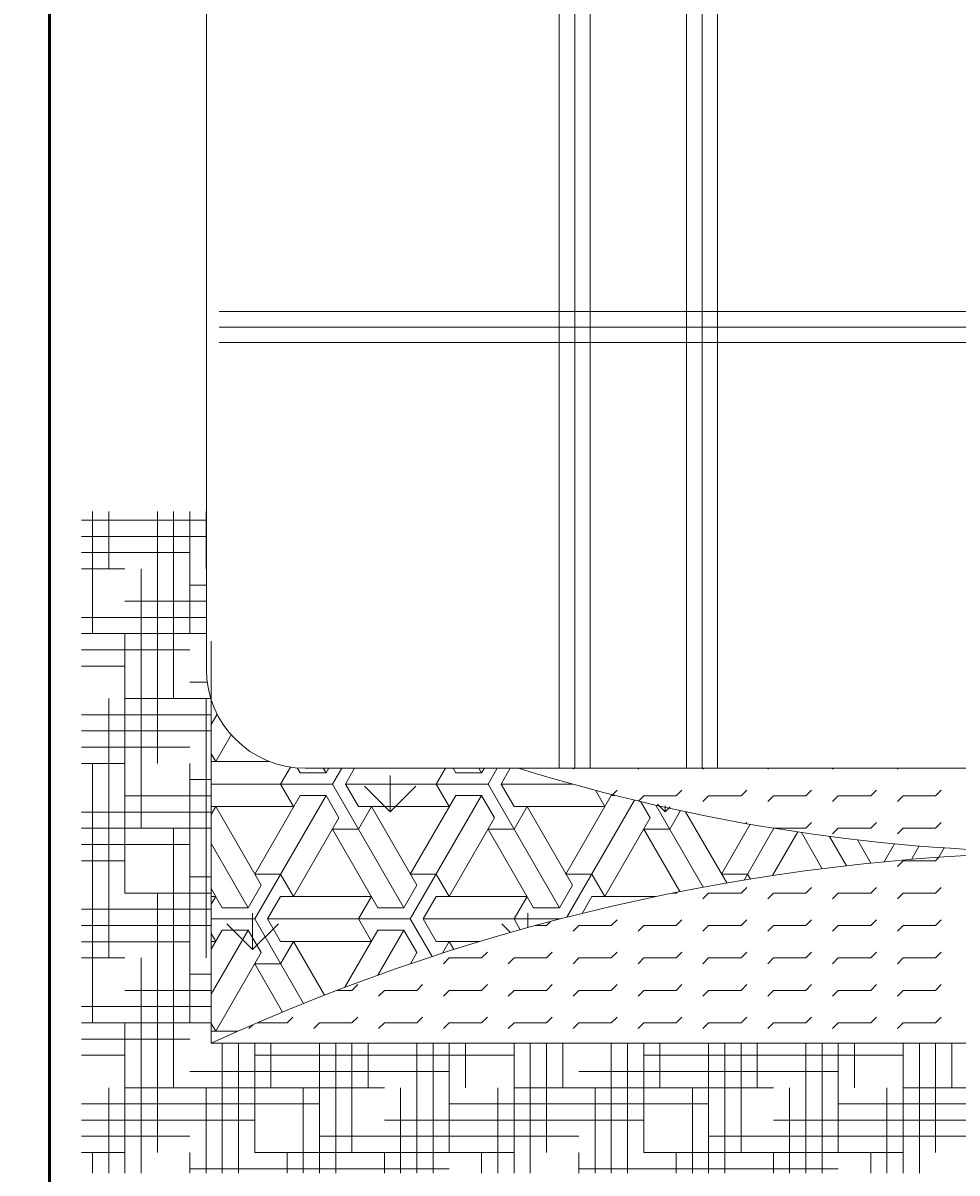
# Model space of a CAD drawing. Units: inches. Extents: x -1517 to -668, y -425 to 52.
# Tile 8 of 13: x -1186 to -1161, y -63 to -32. Entities that reach past the tile are written whole.
import ezdxf

# ---------------------------------------------------------------- set-up
doc = ezdxf.new("R2010")
doc.units = ezdxf.units.IN
doc.header["$MEASUREMENT"] = 0
for name, color, linetype, lineweight in [('A-ANNO-DIMS', 2, 'Continuous', 18), ('furniture block', 8, 'Continuous', 18), ('walls', 240, 'Continuous', 50)]:
    doc.layers.add(name, color=color, linetype=linetype, lineweight=lineweight)
doc.styles.get("Standard").update_dxf_attribs({"font": 'arial.ttf'})
doc.dimstyles.get("Standard").update_dxf_attribs({"dimtxt": 0.18, "dimasz": 0.18, "dimexe": 0.18, "dimexo": 0.0625, "dimgap": 0.09, "dimtad": 0, "dimtih": 1, "dimtoh": 1, "dimdec": 4, "dimzin": 0, "dimdsep": 46, "dimlunit": 4, "dimtxsty": 'Standard', "dimcen": 0.09, "dimadec": 0, "dimazin": 0, "dimtfac": 1, "dimtdec": 4, "dimtofl": 0, "dimtmove": 0, "dimatfit": 3, "dimfxl": 1, "dimtolj": 1, "dimtzin": 0, "dimarcsym": 0})

# ---------------------------------------------------------------- blocks, each defined once
blk = doc.blocks.new('A$C62731D1C')
for p, q in [((0.09627, 0.38824, 0.68571), (0.09627, 2.14084, 0.68571)), ((0.46643, 1.44371, 0.68571), (0.46643, 0.31204, 0.68571)), ((0.47843, 1.44371, 0.68571), (0.47843, 0.31204, 0.68571)), ((0.49043, 1.44371, 0.68571), (0.49043, 0.31204, 0.68571)), ((0.36826, 1.4076, 0.68571), (0.36826, 0.31204, 0.68571)), ((0.38026, 1.4076, 0.68571), (0.38026, 0.31204, 0.68571)), ((0.39226, 1.4076, 0.68571), (0.39226, 0.31204, 0.68571)), ((0.10613, 0.66415, 0.68571), (1.46095, 0.66415, 0.68571)), ((0.10613, 0.65215, 0.68571), (1.46095, 0.65215, 0.68571)), ((0.10613, 0.64015, 0.68571), (1.46095, 0.64015, 0.68571)), ((0.0085, 0.41577, 0.68571), (0.0085, 0.50998, 0.68571)), ((0.021, 0.46577, 0.68571), (0.021, 0.50998, 0.68571)), ((0.0585, 0.31577, 0.68571), (0.0585, 0.50998, 0.68571)), ((0.071, 0.36577, 0.68571), (0.071, 0.50998, 0.68571)), ((0.0835, 0.41577, 0.68571), (0.0835, 0.50998, 0.68571)), ((0.096, 0.46577, 0.68571), (0.096, 0.50998, 0.68571)), ((0, 0.50327, 0.68571), (0.09627, 0.50327, 0.68571)), ((0, 0.49077, 0.68571), (0.09627, 0.49077, 0.68571)), ((0, 0.47827, 0.68571), (0.0835, 0.47827, 0.68571)), ((0, 0.46577, 0.68571), (0.0335, 0.46577, 0.68571)), ((0.046, 0.26577, 0.68571), (0.046, 0.46577, 0.68571)), ((0.0835, 0.45327, 0.68571), (0.09627, 0.45327, 0.68571)), ((0.0335, 0.44077, 0.68571), (0.09627, 0.44077, 0.68571)), ((0, 0.42827, 0.68571), (0.09627, 0.42827, 0.68571)), ((0, 0.41577, 0.68571), (0.09627, 0.41577, 0.68571)), ((0.0335, 0.21577, 0.68571), (0.0335, 0.41577, 0.68571)), ((0.1, 0.1, 0.68571), (0.1, 0.40998, 0.68571)), ((0, 0.40327, 0.68571), (0.0835, 0.40327, 0.68571)), ((0, 0.39077, 0.68571), (0.0335, 0.39077, 0.68571)), ((0.0835, 0.37827, 0.68571), (0.09693, 0.37827, 0.68571)), ((0.021, 0.16577, 0.68571), (0.021, 0.36577, 0.68571)), ((0.0335, 0.36577, 0.68571), (0.09966, 0.36577, 0.68571)), ((0.096, 0.16577, 0.68571), (0.096, 0.36577, 0.68571)), ((0, 0.35327, 0.68571), (0.1, 0.35327, 0.68571)), ((0.1, 0.34567, 0.68571), (0.10459, 0.35362, 0.68571)), ((0, 0.34077, 0.68571), (0.1, 0.34077, 0.68571)), ((0.11542, 0.33773, 0.68571), (0.1035, 0.31709, 0.68571)), ((0, 0.32827, 0.68571), (0.0835, 0.32827, 0.68571)), ((0.1, 0.32316, 0.68571), (0.1035, 0.31709, 0.68571)), ((0, 0.31577, 0.68571), (0.0335, 0.31577, 0.68571)), ((0.0085, 0.11577, 0.68571), (0.0085, 0.31577, 0.68571)), ((0.0835, 0.11577, 0.68571), (0.0835, 0.31577, 0.68571)), ((0.1, 0.31709, 0.68571), (0.14518, 0.31709, 0.68571)), ((0.1535, 0.29977, 0.68571), (0.16108, 0.3129, 0.68571)), ((0.1685, 0.30843, 0.68571), (0.16627, 0.31229, 0.68571)), ((1.39167, 0.31204, 0.68571), (0.17247, 0.31204, 0.68571)), ((0.18642, 0.31204, 0.68571), (0.1885, 0.30843, 0.68571)), ((0.1885, 0.30843, 0.68571), (0.19058, 0.31204, 0.68571)), ((0.1935, 0.29977, 0.68571), (0.20058, 0.31204, 0.68571)), ((0.2035, 0.29977, 0.68571), (0.21058, 0.31204, 0.68571)), ((0.2735, 0.29977, 0.68571), (0.28058, 0.31204, 0.68571)), ((0.2885, 0.30843, 0.68571), (0.28642, 0.31204, 0.68571)), ((0.30642, 0.31204, 0.68571), (0.3085, 0.30843, 0.68571)), ((0.3085, 0.30843, 0.68571), (0.31058, 0.31204, 0.68571)), ((0.3135, 0.29977, 0.68571), (0.32058, 0.31204, 0.68571)), ((0.3235, 0.29977, 0.68571), (0.33058, 0.31204, 0.68571)), ((0.37908, 0.31135, 0.68571), (0.37977, 0.31204, 0.68571)), ((0.42908, 0.31135, 0.68571), (0.42977, 0.31204, 0.68571)), ((0.47908, 0.31135, 0.68571), (0.47977, 0.31204, 0.68571)), ((0.52908, 0.31135, 0.68571), (0.52977, 0.31204, 0.68571)), ((0.57908, 0.31135, 0.68571), (0.57977, 0.31204, 0.68571)), ((0.62908, 0.31135, 0.68571), (0.62977, 0.31204, 0.68571)), ((0.0835, 0.30327, 0.68571), (0.1, 0.30327, 0.68571)), ((0.1885, 0.30843, 0.68571), (0.1685, 0.30843, 0.68571)), ((0.23796, 0.2783, 0.68571), (0.23796, 0.30643, 0.68571)), ((0.3085, 0.30843, 0.68571), (0.2885, 0.30843, 0.68571)), ((0.1935, 0.29977, 0.68571), (0.1, 0.29977, 0.68571)), ((0.1535, 0.29977, 0.68571), (0.1635, 0.28245, 0.68571)), ((0.1935, 0.29977, 0.68571), (0.2485, 0.20451, 0.68571)), ((0.3135, 0.29977, 0.68571), (0.2035, 0.29977, 0.68571)), ((0.2035, 0.29977, 0.68571), (0.2135, 0.28245, 0.68571)), ((0.23796, 0.2783, 0.68571), (0.21807, 0.29819, 0.68571)), ((0.23796, 0.2783, 0.68571), (0.25785, 0.29819, 0.68571)), ((0.2735, 0.29977, 0.68571), (0.2835, 0.28245, 0.68571)), ((0.3135, 0.29977, 0.68571), (0.3685, 0.20451, 0.68571)), ((0.37861, 0.29977, 0.68571), (0.3235, 0.29977, 0.68571)), ((0.3235, 0.29977, 0.68571), (0.3335, 0.28245, 0.68571)), ((0.39626, 0.295, 0.68571), (0.4035, 0.28245, 0.68571)), ((0.40934, 0.29161, 0.68571), (0.41292, 0.29519, 0.68571)), ((0.4585, 0.29077, 0.68571), (0.46292, 0.29519, 0.68571)), ((0.5085, 0.29077, 0.68571), (0.51292, 0.29519, 0.68571)), ((0.5585, 0.29077, 0.68571), (0.56292, 0.29519, 0.68571)), ((0.6085, 0.29077, 0.68571), (0.61292, 0.29519, 0.68571)), ((0.6585, 0.29077, 0.68571), (0.66292, 0.29519, 0.68571)), ((0.0335, 0.29077, 0.68571), (0.1, 0.29077, 0.68571)), ((0.1335, 0.19585, 0.68571), (0.1885, 0.29111, 0.68571)), ((0.1685, 0.29111, 0.68571), (0.1335, 0.23049, 0.68571)), ((0.1885, 0.29111, 0.68571), (0.1685, 0.29111, 0.68571)), ((0.1885, 0.29111, 0.68571), (0.1985, 0.27379, 0.68571)), ((0.2535, 0.19585, 0.68571), (0.3085, 0.29111, 0.68571)), ((0.2885, 0.29111, 0.68571), (0.2535, 0.23049, 0.68571)), ((0.3085, 0.29111, 0.68571), (0.2885, 0.29111, 0.68571)), ((0.3085, 0.29111, 0.68571), (0.3185, 0.27379, 0.68571)), ((0.4085, 0.29111, 0.68571), (0.3735, 0.23049, 0.68571)), ((0.37428, 0.19721, 0.68571), (0.42636, 0.2874, 0.68571)), ((0.4113, 0.29111, 0.68571), (0.4085, 0.29111, 0.68571)), ((0.4294, 0.28667, 0.68571), (0.4335, 0.29077, 0.68571)), ((0.43133, 0.28621, 0.68571), (0.4385, 0.27379, 0.68571)), ((0.4335, 0.29077, 0.68571), (0.4585, 0.29077, 0.68571)), ((0.45009, 0.2783, 0.68571), (0.44401, 0.28439, 0.68571)), ((0.47908, 0.28635, 0.68571), (0.4835, 0.29077, 0.68571)), ((0.4835, 0.29077, 0.68571), (0.5085, 0.29077, 0.68571)), ((0.52908, 0.28635, 0.68571), (0.5335, 0.29077, 0.68571)), ((0.5335, 0.29077, 0.68571), (0.5585, 0.29077, 0.68571)), ((0.57908, 0.28635, 0.68571), (0.5835, 0.29077, 0.68571)), ((0.5835, 0.29077, 0.68571), (0.6085, 0.29077, 0.68571)), ((0.62908, 0.28635, 0.68571), (0.6335, 0.29077, 0.68571)), ((0.6335, 0.29077, 0.68571), (0.6585, 0.29077, 0.68571)), ((0, 0.27827, 0.68571), (0.1, 0.27827, 0.68571)), ((0.1, 0.27639, 0.68571), (0.1035, 0.28245, 0.68571)), ((0.1, 0.28245, 0.68571), (0.1635, 0.28245, 0.68571)), ((0.1385, 0.22183, 0.68571), (0.1035, 0.28245, 0.68571)), ((0.2135, 0.26513, 0.68571), (0.2235, 0.28245, 0.68571)), ((0.2135, 0.28245, 0.68571), (0.2835, 0.28245, 0.68571)), ((0.2585, 0.22183, 0.68571), (0.2235, 0.28245, 0.68571)), ((0.3335, 0.26513, 0.68571), (0.3435, 0.28245, 0.68571)), ((0.3335, 0.28245, 0.68571), (0.4035, 0.28245, 0.68571)), ((0.3785, 0.22183, 0.68571), (0.3435, 0.28245, 0.68571)), ((0.44289, 0.28352, 0.68571), (0.47937, 0.22033, 0.68571)), ((0.45009, 0.2783, 0.68571), (0.45009, 0.28301, 0.68571)), ((0.45009, 0.2783, 0.68571), (0.45394, 0.28215, 0.68571)), ((0.4535, 0.26513, 0.68571), (0.46171, 0.27934, 0.68571)), ((0.49749, 0.22358, 0.68571), (0.4658, 0.27847, 0.68571)), ((0.1985, 0.27379, 0.68571), (0.1635, 0.21317, 0.68571)), ((0.3185, 0.27379, 0.68571), (0.2835, 0.21317, 0.68571)), ((0.4385, 0.27379, 0.68571), (0.4035, 0.21317, 0.68571)), ((0.51564, 0.26884, 0.68571), (0.4935, 0.23049, 0.68571)), ((0.51218, 0.26945, 0.68571), (0.51292, 0.27019, 0.68571)), ((0.5585, 0.26577, 0.68571), (0.56292, 0.27019, 0.68571)), ((0.6085, 0.26577, 0.68571), (0.61292, 0.27019, 0.68571)), ((0.6585, 0.26577, 0.68571), (0.66292, 0.27019, 0.68571)), ((0, 0.26577, 0.68571), (0.1, 0.26577, 0.68571)), ((0.071, 0.06577, 0.68571), (0.071, 0.26577, 0.68571)), ((0.2135, 0.26513, 0.68571), (0.1935, 0.26513, 0.68571)), ((0.2285, 0.20451, 0.68571), (0.1935, 0.26513, 0.68571)), ((0.3335, 0.26513, 0.68571), (0.3135, 0.26513, 0.68571)), ((0.3485, 0.20451, 0.68571), (0.3135, 0.26513, 0.68571)), ((0.4535, 0.26513, 0.68571), (0.4335, 0.26513, 0.68571)), ((0.46136, 0.21689, 0.68571), (0.4335, 0.26513, 0.68571)), ((0.51081, 0.22583, 0.68571), (0.53387, 0.26577, 0.68571)), ((0.55222, 0.26292, 0.68571), (0.53281, 0.2293, 0.68571)), ((0.53385, 0.26577, 0.68571), (0.5585, 0.26577, 0.68571)), ((0.57113, 0.2346, 0.68571), (0.55502, 0.2625, 0.68571)), ((0.57677, 0.25948, 0.68571), (0.58983, 0.23685, 0.68571)), ((0.57908, 0.26135, 0.68571), (0.5835, 0.26577, 0.68571)), ((0.5835, 0.26577, 0.68571), (0.6085, 0.26577, 0.68571)), ((0.62908, 0.26135, 0.68571), (0.6335, 0.26577, 0.68571)), ((0.6335, 0.26577, 0.68571), (0.6585, 0.26577, 0.68571)), ((0, 0.25327, 0.68571), (0.0835, 0.25327, 0.68571)), ((0.1, 0.25388, 0.68571), (0.1285, 0.20451, 0.68571)), ((0.60866, 0.23889, 0.68571), (0.5983, 0.25682, 0.68571)), ((0.62695, 0.25378, 0.68571), (0.61894, 0.2399, 0.68571)), ((0.64002, 0.24179, 0.68571), (0.64597, 0.25209, 0.68571)), ((0.66513, 0.25064, 0.68571), (0.66094, 0.24338, 0.68571)), ((0, 0.24077, 0.68571), (0.0335, 0.24077, 0.68571)), ((0.62908, 0.23635, 0.68571), (0.6335, 0.24077, 0.68571)), ((0.6335, 0.24077, 0.68571), (0.6585, 0.24077, 0.68571)), ((0.6585, 0.24077, 0.68571), (0.66112, 0.24339, 0.68571)), ((0.0835, 0.22827, 0.68571), (0.1, 0.22827, 0.68571)), ((0.1285, 0.20451, 0.68571), (0.1385, 0.22183, 0.68571)), ((0.1535, 0.23049, 0.68571), (0.1335, 0.23049, 0.68571)), ((0.1535, 0.23049, 0.68571), (0.1635, 0.21317, 0.68571)), ((0.2485, 0.20451, 0.68571), (0.2585, 0.22183, 0.68571)), ((0.2735, 0.23049, 0.68571), (0.2535, 0.23049, 0.68571)), ((0.2735, 0.23049, 0.68571), (0.2835, 0.21317, 0.68571)), ((0.3685, 0.20451, 0.68571), (0.3785, 0.22183, 0.68571)), ((0.3935, 0.23049, 0.68571), (0.3735, 0.23049, 0.68571)), ((0.3935, 0.23049, 0.68571), (0.4035, 0.21317, 0.68571)), ((0.5135, 0.23049, 0.68571), (0.4935, 0.23049, 0.68571)), ((0.5135, 0.23049, 0.68571), (0.51573, 0.22663, 0.68571)), ((0.0335, 0.21577, 0.68571), (0.1, 0.21577, 0.68571)), ((0.0585, 0.01577, 0.68571), (0.0585, 0.21577, 0.68571)), ((0.1085, 0.20451, 0.68571), (0.1, 0.21924, 0.68571)), ((0.1, 0.20711, 0.68571), (0.1035, 0.21317, 0.68571)), ((0.1, 0.21317, 0.68571), (0.1035, 0.21317, 0.68571)), ((0.1435, 0.19585, 0.68571), (0.1535, 0.21317, 0.68571)), ((0.1535, 0.21317, 0.68571), (0.2235, 0.21317, 0.68571)), ((0.2135, 0.19585, 0.68571), (0.2235, 0.21317, 0.68571)), ((0.2635, 0.19585, 0.68571), (0.2735, 0.21317, 0.68571)), ((0.2735, 0.21317, 0.68571), (0.3435, 0.21317, 0.68571)), ((0.3335, 0.19585, 0.68571), (0.3435, 0.21317, 0.68571)), ((0.38598, 0.20015, 0.68571), (0.3935, 0.21317, 0.68571)), ((0.3935, 0.21317, 0.68571), (0.44307, 0.21317, 0.68571)), ((0.45574, 0.21577, 0.68571), (0.4585, 0.21577, 0.68571)), ((0.4585, 0.21577, 0.68571), (0.45919, 0.21646, 0.68571)), ((0.47908, 0.21135, 0.68571), (0.4835, 0.21577, 0.68571)), ((0.4835, 0.21577, 0.68571), (0.5085, 0.21577, 0.68571)), ((0.5085, 0.21577, 0.68571), (0.51292, 0.22019, 0.68571)), ((0.52908, 0.21135, 0.68571), (0.5335, 0.21577, 0.68571)), ((0.5335, 0.21577, 0.68571), (0.5585, 0.21577, 0.68571)), ((0.5585, 0.21577, 0.68571), (0.56292, 0.22019, 0.68571)), ((0.57908, 0.21135, 0.68571), (0.5835, 0.21577, 0.68571)), ((0.5835, 0.21577, 0.68571), (0.6085, 0.21577, 0.68571)), ((0.6085, 0.21577, 0.68571), (0.61292, 0.22019, 0.68571)), ((0.62908, 0.21135, 0.68571), (0.6335, 0.21577, 0.68571)), ((0.6335, 0.21577, 0.68571), (0.6585, 0.21577, 0.68571)), ((0.6585, 0.21577, 0.68571), (0.66292, 0.22019, 0.68571)), ((0.1285, 0.20451, 0.68571), (0.1085, 0.20451, 0.68571)), ((0.2485, 0.20451, 0.68571), (0.2285, 0.20451, 0.68571)), ((0.3685, 0.20451, 0.68571), (0.3485, 0.20451, 0.68571)), ((0, 0.20327, 0.68571), (0.1, 0.20327, 0.68571)), ((0.1335, 0.19585, 0.68571), (0.1, 0.19585, 0.68571)), ((0.13189, 0.17223, 0.68571), (0.13189, 0.20036, 0.68571)), ((0.1335, 0.19585, 0.68571), (0.17113, 0.13067, 0.68571)), ((0.2535, 0.19585, 0.68571), (0.1435, 0.19585, 0.68571)), ((0.1435, 0.19585, 0.68571), (0.1535, 0.17853, 0.68571)), ((0.2135, 0.19585, 0.68571), (0.2235, 0.17853, 0.68571)), ((0.2535, 0.19585, 0.68571), (0.27024, 0.16687, 0.68571)), ((0.36902, 0.19585, 0.68571), (0.2635, 0.19585, 0.68571)), ((0.2635, 0.19585, 0.68571), (0.2735, 0.17853, 0.68571)), ((0.3335, 0.19585, 0.68571), (0.33829, 0.18757, 0.68571)), ((0.34403, 0.18916, 0.68571), (0.34403, 0.20036, 0.68571)), ((0.4085, 0.19077, 0.68571), (0.41292, 0.19519, 0.68571)), ((0.4585, 0.19077, 0.68571), (0.46292, 0.19519, 0.68571)), ((0.5085, 0.19077, 0.68571), (0.51292, 0.19519, 0.68571)), ((0.5585, 0.19077, 0.68571), (0.56292, 0.19519, 0.68571)), ((0.6085, 0.19077, 0.68571), (0.61292, 0.19519, 0.68571)), ((0.6585, 0.19077, 0.68571), (0.66292, 0.19519, 0.68571)), ((0, 0.19077, 0.68571), (0.1, 0.19077, 0.68571)), ((0.1, 0.13782, 0.68571), (0.1285, 0.18719, 0.68571)), ((0.1085, 0.18719, 0.68571), (0.1, 0.17247, 0.68571)), ((0.1285, 0.18719, 0.68571), (0.1085, 0.18719, 0.68571)), ((0.13189, 0.17223, 0.68571), (0.11201, 0.19212, 0.68571)), ((0.1285, 0.18719, 0.68571), (0.1385, 0.16987, 0.68571)), ((0.13189, 0.17223, 0.68571), (0.15178, 0.19212, 0.68571)), ((0.2285, 0.18719, 0.68571), (0.20307, 0.14314, 0.68571)), ((0.22848, 0.15251, 0.68571), (0.2485, 0.18719, 0.68571)), ((0.2485, 0.18719, 0.68571), (0.2285, 0.18719, 0.68571)), ((0.2485, 0.18719, 0.68571), (0.2585, 0.16987, 0.68571)), ((0.33081, 0.18545, 0.68571), (0.32414, 0.19212, 0.68571)), ((0.34988, 0.19077, 0.68571), (0.3585, 0.19077, 0.68571)), ((0.3585, 0.19077, 0.68571), (0.36166, 0.19393, 0.68571)), ((0.37908, 0.18635, 0.68571), (0.3835, 0.19077, 0.68571)), ((0.3835, 0.19077, 0.68571), (0.4085, 0.19077, 0.68571)), ((0.42908, 0.18635, 0.68571), (0.4335, 0.19077, 0.68571)), ((0.4335, 0.19077, 0.68571), (0.4585, 0.19077, 0.68571)), ((0.47908, 0.18635, 0.68571), (0.4835, 0.19077, 0.68571)), ((0.4835, 0.19077, 0.68571), (0.5085, 0.19077, 0.68571)), ((0.52908, 0.18635, 0.68571), (0.5335, 0.19077, 0.68571)), ((0.5335, 0.19077, 0.68571), (0.5585, 0.19077, 0.68571)), ((0.57908, 0.18635, 0.68571), (0.5835, 0.19077, 0.68571)), ((0.5835, 0.19077, 0.68571), (0.6085, 0.19077, 0.68571)), ((0.62908, 0.18635, 0.68571), (0.6335, 0.19077, 0.68571)), ((0.6335, 0.19077, 0.68571), (0.6585, 0.19077, 0.68571)), ((0, 0.17827, 0.68571), (0.0835, 0.17827, 0.68571)), ((0.1, 0.1846, 0.68571), (0.1035, 0.17853, 0.68571)), ((0.1, 0.17853, 0.68571), (0.1035, 0.17853, 0.68571)), ((0.1535, 0.16121, 0.68571), (0.1635, 0.17853, 0.68571)), ((0.1535, 0.17853, 0.68571), (0.2235, 0.17853, 0.68571)), ((0.18741, 0.13712, 0.68571), (0.1635, 0.17853, 0.68571)), ((0.2735, 0.17853, 0.68571), (0.30724, 0.17853, 0.68571)), ((0.27828, 0.16948, 0.68571), (0.2835, 0.17853, 0.68571)), ((0.2871, 0.1723, 0.68571), (0.2835, 0.17853, 0.68571)), ((0.1385, 0.16987, 0.68571), (0.1035, 0.10925, 0.68571)), ((0.2585, 0.16987, 0.68571), (0.25354, 0.16128, 0.68571)), ((0.3085, 0.16577, 0.68571), (0.31292, 0.17019, 0.68571)), ((0.3585, 0.16577, 0.68571), (0.36292, 0.17019, 0.68571)), ((0.4085, 0.16577, 0.68571), (0.41292, 0.17019, 0.68571)), ((0.4585, 0.16577, 0.68571), (0.46292, 0.17019, 0.68571)), ((0.5085, 0.16577, 0.68571), (0.51292, 0.17019, 0.68571)), ((0.5585, 0.16577, 0.68571), (0.56292, 0.17019, 0.68571)), ((0.6085, 0.16577, 0.68571), (0.61292, 0.17019, 0.68571)), ((0.6585, 0.16577, 0.68571), (0.66292, 0.17019, 0.68571)), ((0, 0.16577, 0.68571), (0.0335, 0.16577, 0.68571)), ((0.046, 0, 0.68571), (0.046, 0.16577, 0.68571)), ((0.1535, 0.16121, 0.68571), (0.1335, 0.16121, 0.68571)), ((0.15496, 0.12405, 0.68571), (0.1335, 0.16121, 0.68571)), ((0.27908, 0.16135, 0.68571), (0.2835, 0.16577, 0.68571)), ((0.2835, 0.16577, 0.68571), (0.3085, 0.16577, 0.68571)), ((0.32908, 0.16135, 0.68571), (0.3335, 0.16577, 0.68571)), ((0.3335, 0.16577, 0.68571), (0.3585, 0.16577, 0.68571)), ((0.37908, 0.16135, 0.68571), (0.3835, 0.16577, 0.68571)), ((0.3835, 0.16577, 0.68571), (0.4085, 0.16577, 0.68571)), ((0.42908, 0.16135, 0.68571), (0.4335, 0.16577, 0.68571)), ((0.4335, 0.16577, 0.68571), (0.4585, 0.16577, 0.68571)), ((0.47908, 0.16135, 0.68571), (0.4835, 0.16577, 0.68571)), ((0.4835, 0.16577, 0.68571), (0.5085, 0.16577, 0.68571)), ((0.52908, 0.16135, 0.68571), (0.5335, 0.16577, 0.68571)), ((0.5335, 0.16577, 0.68571), (0.5585, 0.16577, 0.68571)), ((0.57908, 0.16135, 0.68571), (0.5835, 0.16577, 0.68571)), ((0.5835, 0.16577, 0.68571), (0.6085, 0.16577, 0.68571)), ((0.62908, 0.16135, 0.68571), (0.6335, 0.16577, 0.68571)), ((0.6335, 0.16577, 0.68571), (0.6585, 0.16577, 0.68571)), ((0.0835, 0.15327, 0.68571), (0.1, 0.15327, 0.68571)), ((0.2085, 0.14077, 0.68571), (0.21292, 0.14519, 0.68571)), ((0.2585, 0.14077, 0.68571), (0.26292, 0.14519, 0.68571)), ((0.3085, 0.14077, 0.68571), (0.31292, 0.14519, 0.68571)), ((0.3585, 0.14077, 0.68571), (0.36292, 0.14519, 0.68571)), ((0.4085, 0.14077, 0.68571), (0.41292, 0.14519, 0.68571)), ((0.4585, 0.14077, 0.68571), (0.46292, 0.14519, 0.68571)), ((0.5085, 0.14077, 0.68571), (0.51292, 0.14519, 0.68571)), ((0.5585, 0.14077, 0.68571), (0.56292, 0.14519, 0.68571)), ((0.6085, 0.14077, 0.68571), (0.61292, 0.14519, 0.68571)), ((0.6585, 0.14077, 0.68571), (0.66292, 0.14519, 0.68571)), ((0.0335, 0.14077, 0.68571), (0.1, 0.14077, 0.68571)), ((0.19684, 0.14077, 0.68571), (0.2085, 0.14077, 0.68571)), ((0.22908, 0.13635, 0.68571), (0.2335, 0.14077, 0.68571)), ((0.2335, 0.14077, 0.68571), (0.2585, 0.14077, 0.68571)), ((0.27908, 0.13635, 0.68571), (0.2835, 0.14077, 0.68571)), ((0.2835, 0.14077, 0.68571), (0.3085, 0.14077, 0.68571)), ((0.32908, 0.13635, 0.68571), (0.3335, 0.14077, 0.68571)), ((0.3335, 0.14077, 0.68571), (0.3585, 0.14077, 0.68571)), ((0.37908, 0.13635, 0.68571), (0.3835, 0.14077, 0.68571)), ((0.3835, 0.14077, 0.68571), (0.4085, 0.14077, 0.68571)), ((0.42908, 0.13635, 0.68571), (0.4335, 0.14077, 0.68571)), ((0.4335, 0.14077, 0.68571), (0.4585, 0.14077, 0.68571)), ((0.47908, 0.13635, 0.68571), (0.4835, 0.14077, 0.68571)), ((0.4835, 0.14077, 0.68571), (0.5085, 0.14077, 0.68571)), ((0.52908, 0.13635, 0.68571), (0.5335, 0.14077, 0.68571)), ((0.5335, 0.14077, 0.68571), (0.5585, 0.14077, 0.68571)), ((0.57908, 0.13635, 0.68571), (0.5835, 0.14077, 0.68571)), ((0.5835, 0.14077, 0.68571), (0.6085, 0.14077, 0.68571)), ((0.62908, 0.13635, 0.68571), (0.6335, 0.14077, 0.68571)), ((0.6335, 0.14077, 0.68571), (0.6585, 0.14077, 0.68571)), ((0, 0.12827, 0.68571), (0.1, 0.12827, 0.68571)), ((0, 0.11577, 0.68571), (0.1, 0.11577, 0.68571)), ((0.0335, 0, 0.68571), (0.0335, 0.11577, 0.68571)), ((0.1, 0.11531, 0.68571), (0.1035, 0.10925, 0.68571)), ((0.1354, 0.11577, 0.68571), (0.1585, 0.11577, 0.68571)), ((0.1585, 0.11577, 0.68571), (0.16292, 0.12019, 0.68571)), ((0.17908, 0.11135, 0.68571), (0.1835, 0.11577, 0.68571)), ((0.1835, 0.11577, 0.68571), (0.2085, 0.11577, 0.68571)), ((0.2085, 0.11577, 0.68571), (0.21292, 0.12019, 0.68571)), ((0.22908, 0.11135, 0.68571), (0.2335, 0.11577, 0.68571)), ((0.2335, 0.11577, 0.68571), (0.2585, 0.11577, 0.68571)), ((0.2585, 0.11577, 0.68571), (0.26292, 0.12019, 0.68571)), ((0.27908, 0.11135, 0.68571), (0.2835, 0.11577, 0.68571)), ((0.2835, 0.11577, 0.68571), (0.3085, 0.11577, 0.68571)), ((0.3085, 0.11577, 0.68571), (0.31292, 0.12019, 0.68571)), ((0.32908, 0.11135, 0.68571), (0.3335, 0.11577, 0.68571)), ((0.3335, 0.11577, 0.68571), (0.3585, 0.11577, 0.68571)), ((0.3585, 0.11577, 0.68571), (0.36292, 0.12019, 0.68571)), ((0.37908, 0.11135, 0.68571), (0.3835, 0.11577, 0.68571)), ((0.3835, 0.11577, 0.68571), (0.4085, 0.11577, 0.68571)), ((0.4085, 0.11577, 0.68571), (0.41292, 0.12019, 0.68571)), ((0.42908, 0.11135, 0.68571), (0.4335, 0.11577, 0.68571)), ((0.4335, 0.11577, 0.68571), (0.4585, 0.11577, 0.68571)), ((0.4585, 0.11577, 0.68571), (0.46292, 0.12019, 0.68571)), ((0.47908, 0.11135, 0.68571), (0.4835, 0.11577, 0.68571)), ((0.4835, 0.11577, 0.68571), (0.5085, 0.11577, 0.68571)), ((0.5085, 0.11577, 0.68571), (0.51292, 0.12019, 0.68571)), ((0.52908, 0.11135, 0.68571), (0.5335, 0.11577, 0.68571)), ((0.5335, 0.11577, 0.68571), (0.5585, 0.11577, 0.68571)), ((0.5585, 0.11577, 0.68571), (0.56292, 0.12019, 0.68571)), ((0.57908, 0.11135, 0.68571), (0.5835, 0.11577, 0.68571)), ((0.5835, 0.11577, 0.68571), (0.6085, 0.11577, 0.68571)), ((0.6085, 0.11577, 0.68571), (0.61292, 0.12019, 0.68571)), ((0.62908, 0.11135, 0.68571), (0.6335, 0.11577, 0.68571)), ((0.6335, 0.11577, 0.68571), (0.6585, 0.11577, 0.68571)), ((0.6585, 0.11577, 0.68571), (0.66292, 0.12019, 0.68571)), ((0.1, 0.10925, 0.68571), (0.12048, 0.10925, 0.68571)), ((0.12908, 0.11135, 0.68571), (0.13206, 0.11432, 0.68571)), ((0, 0.10327, 0.68571), (0.0835, 0.10327, 0.68571)), ((1.44488, 0.1, 0.68571), (0.1, 0.1, 0.68571)), ((0.1085, 0, 0.68571), (0.1085, 0.1, 0.68571)), ((0.121, 0, 0.68571), (0.121, 0.1, 0.68571)), ((0.1335, 0.01577, 0.68571), (0.1335, 0.1, 0.68571)), ((0.146, 0.06577, 0.68571), (0.146, 0.1, 0.68571)), ((0.1835, 0, 0.68571), (0.1835, 0.1, 0.68571)), ((0.196, 0, 0.68571), (0.196, 0.1, 0.68571)), ((0.2085, 0.01577, 0.68571), (0.2085, 0.1, 0.68571)), ((0.221, 0.06577, 0.68571), (0.221, 0.1, 0.68571)), ((0.2585, 0, 0.68571), (0.2585, 0.1, 0.68571)), ((0.271, 0, 0.68571), (0.271, 0.1, 0.68571)), ((0.2835, 0.01577, 0.68571), (0.2835, 0.1, 0.68571)), ((0.296, 0.06577, 0.68571), (0.296, 0.1, 0.68571)), ((0.3335, 0, 0.68571), (0.3335, 0.1, 0.68571)), ((0.346, 0, 0.68571), (0.346, 0.1, 0.68571)), ((0.3585, 0.01577, 0.68571), (0.3585, 0.1, 0.68571)), ((0.371, 0.06577, 0.68571), (0.371, 0.1, 0.68571)), ((0.4085, 0, 0.68571), (0.4085, 0.1, 0.68571)), ((0.421, 0, 0.68571), (0.421, 0.1, 0.68571)), ((0.4335, 0.01577, 0.68571), (0.4335, 0.1, 0.68571)), ((0.446, 0.06577, 0.68571), (0.446, 0.1, 0.68571)), ((0.4835, 0, 0.68571), (0.4835, 0.1, 0.68571)), ((0.496, 0, 0.68571), (0.496, 0.1, 0.68571)), ((0.5085, 0.01577, 0.68571), (0.5085, 0.1, 0.68571)), ((0.521, 0.06577, 0.68571), (0.521, 0.1, 0.68571)), ((0.5585, 0, 0.68571), (0.5585, 0.1, 0.68571)), ((0.571, 0, 0.68571), (0.571, 0.1, 0.68571)), ((0.5835, 0.01577, 0.68571), (0.5835, 0.1, 0.68571)), ((0.596, 0.06577, 0.68571), (0.596, 0.1, 0.68571)), ((0.6335, 0, 0.68571), (0.6335, 0.1, 0.68571)), ((0.646, 0, 0.68571), (0.646, 0.1, 0.68571)), ((0.6585, 0.01577, 0.68571), (0.6585, 0.1, 0.68571)), ((0.671, 0.06577, 0.68571), (0.671, 0.1, 0.68571)), ((0, 0.09077, 0.68571), (0.0335, 0.09077, 0.68571)), ((0.1335, 0.09077, 0.68571), (0.3335, 0.09077, 0.68571)), ((0.4335, 0.09077, 0.68571), (0.6335, 0.09077, 0.68571)), ((0.0835, 0.07827, 0.68571), (0.2835, 0.07827, 0.68571)), ((0.3835, 0.07827, 0.68571), (0.5835, 0.07827, 0.68571)), ((0.021, 0, 0.68571), (0.021, 0.06577, 0.68571)), ((0.0335, 0.06577, 0.68571), (0.2335, 0.06577, 0.68571)), ((0.096, 0, 0.68571), (0.096, 0.06577, 0.68571)), ((0.171, 0, 0.68571), (0.171, 0.06577, 0.68571)), ((0.246, 0, 0.68571), (0.246, 0.06577, 0.68571)), ((0.321, 0, 0.68571), (0.321, 0.06577, 0.68571)), ((0.3335, 0.06577, 0.68571), (0.5335, 0.06577, 0.68571)), ((0.396, 0, 0.68571), (0.396, 0.06577, 0.68571)), ((0.471, 0, 0.68571), (0.471, 0.06577, 0.68571)), ((0.546, 0, 0.68571), (0.546, 0.06577, 0.68571)), ((0.621, 0, 0.68571), (0.621, 0.06577, 0.68571)), ((0.6335, 0.06577, 0.68571), (0.8335, 0.06577, 0.68571)), ((0, 0.05327, 0.68571), (0.1835, 0.05327, 0.68571)), ((0.2835, 0.05327, 0.68571), (0.4835, 0.05327, 0.68571)), ((0.5835, 0.05327, 0.68571), (0.7835, 0.05327, 0.68571)), ((0, 0.04077, 0.68571), (0.1335, 0.04077, 0.68571)), ((0.2335, 0.04077, 0.68571), (0.4335, 0.04077, 0.68571)), ((0.5335, 0.04077, 0.68571), (0.7335, 0.04077, 0.68571)), ((0, 0.02827, 0.68571), (0.0835, 0.02827, 0.68571)), ((0.1835, 0.02827, 0.68571), (0.3835, 0.02827, 0.68571)), ((0.4835, 0.02827, 0.68571), (0.6835, 0.02827, 0.68571)), ((0, 0.01577, 0.68571), (0.0335, 0.01577, 0.68571)), ((0.0085, 0, 0.68571), (0.0085, 0.01577, 0.68571)), ((0.0835, 0, 0.68571), (0.0835, 0.01577, 0.68571)), ((0.1335, 0.01577, 0.68571), (0.3335, 0.01577, 0.68571)), ((0.1585, 0, 0.68571), (0.1585, 0.01577, 0.68571)), ((0.2335, 0, 0.68571), (0.2335, 0.01577, 0.68571)), ((0.3085, 0, 0.68571), (0.3085, 0.01577, 0.68571)), ((0.3835, 0, 0.68571), (0.3835, 0.01577, 0.68571)), ((0.4335, 0.01577, 0.68571), (0.6335, 0.01577, 0.68571)), ((0.4585, 0, 0.68571), (0.4585, 0.01577, 0.68571)), ((0.5335, 0, 0.68571), (0.5335, 0.01577, 0.68571)), ((0.6085, 0, 0.68571), (0.6085, 0.01577, 0.68571)), ((0.0835, 0.00327, 0.68571), (0.2835, 0.00327, 0.68571)), ((0.3835, 0.00327, 0.68571), (0.5835, 0.00327, 0.68571))]:
    blk.add_line(p, q)
for centre, radius, start, end in [((0.17247, 0.38824, 0.68571), 0.0762, 180, 270), ((0.76456, 1.69033, 0.68571), 1.44313, 252.76056, 287.23944), ((0.77244, -1.36185, 0.68571), 1.6091, 65.29791, 114.70209)]:
    blk.add_arc(centre, radius, start, end)
blk = doc.blocks.new('A$C0E6D7E3D')
blk.add_blockref('A$C62731D1C', (0, 0))
blk = doc.blocks.new('*D53')
at = {"layer": 'A-ANNO-DIMS', "color": 0, "lineweight": -2, "transparency": 16777216}
for p, q in [((-1242.504, -153.307), (-1242.504, 52.11)), ((-1242.324, 51.93), (-1128.794, 51.93)), ((-1014.684, 51.93), (-1128.213, 51.93)), ((-1014.504, -150.307), (-1014.504, 52.11))]:
    blk.add_line(p, q, dxfattribs=at)
at = {"layer": 'A-ANNO-DIMS', "color": 0, "transparency": 16777216}
for points in [[(-1242.324, 51.96), (-1242.324, 51.9), (-1242.504, 51.93)], [(-1014.684, 51.96), (-1014.684, 51.9), (-1014.504, 51.93)]]:
    blk.add_solid(points, dxfattribs=at)
at = {"layer": 'Defpoints', "color": 0, "transparency": 16777216}
for p in [(-1014.504, 51.93), (-1014.504, -150.37), (-1242.504, -153.37)]:
    blk.add_point(p, dxfattribs=at)
at = {"layer": 'A-ANNO-DIMS', "color": 0, "transparency": 16777216, "insert": (-1128.504, 51.93), "char_height": 0.18, "attachment_point": 5}
blk.add_mtext('\\A1;228', dxfattribs=at)
blk = doc.blocks.new('*D72')
at = {"layer": 'A-ANNO-DIMS', "color": 0, "lineweight": -2, "transparency": 16777216}
for p, q in [((-1285.841, -16.282), (-980.024, -16.282)), ((-980.204, -16.462), (-980.204, -59.144)), ((-980.204, -102.19), (-980.204, -59.508)), ((-1285.841, -102.37), (-980.024, -102.37))]:
    blk.add_line(p, q, dxfattribs=at)
at = {"layer": 'A-ANNO-DIMS', "color": 0, "transparency": 16777216}
for points in [[(-980.234, -16.462), (-980.174, -16.462), (-980.204, -16.282)], [(-980.234, -102.19), (-980.174, -102.19), (-980.204, -102.37)]]:
    blk.add_solid(points, dxfattribs=at)
at = {"layer": 'Defpoints', "color": 0, "transparency": 16777216}
for p in [(-1285.904, -16.282), (-1285.904, -102.37), (-980.204, -102.37)]:
    blk.add_point(p, dxfattribs=at)
at = {"layer": 'A-ANNO-DIMS', "color": 0, "transparency": 16777216, "insert": (-980.204, -59.326), "char_height": 0.18, "attachment_point": 5}
blk.add_mtext('\\A1;86.09', dxfattribs=at)
blk = doc.blocks.new('*D73')
at = {"layer": 'A-ANNO-DIMS', "color": 0, "lineweight": -2, "transparency": 16777216}
for p, q in [((-1089.366, -16.37), (-1516.984, -16.37)), ((-1516.804, -16.55), (-1516.804, -59.188)), ((-1516.804, -102.19), (-1516.804, -59.552)), ((-1089.366, -102.37), (-1516.984, -102.37))]:
    blk.add_line(p, q, dxfattribs=at)
at = {"layer": 'A-ANNO-DIMS', "color": 0, "transparency": 16777216}
for points in [[(-1516.834, -16.55), (-1516.774, -16.55), (-1516.804, -16.37)], [(-1516.834, -102.19), (-1516.774, -102.19), (-1516.804, -102.37)]]:
    blk.add_solid(points, dxfattribs=at)
at = {"layer": 'Defpoints', "color": 0, "transparency": 16777216}
for p in [(-1089.304, -16.37), (-1516.804, -102.37), (-1089.304, -102.37)]:
    blk.add_point(p, dxfattribs=at)
at = {"layer": 'A-ANNO-DIMS', "color": 0, "transparency": 16777216, "insert": (-1516.804, -59.37), "char_height": 0.18, "attachment_point": 5}
blk.add_mtext('\\A1;86', dxfattribs=at)

msp = doc.modelspace()

# ---------------------------------------------------------------- linework, layer by layer
at = {"layer": 'walls'}
msp.add_line((-1185.3037, -102.37), (-1185.3037, 17.63), dxfattribs=at)

# ---------------------------------------------------------------- block references
at = {"layer": 'furniture block', "xscale": 34.99562554665724, "yscale": 34.99562554665724, "zscale": 34.99562554665724}
msp.add_blockref('A$C0E6D7E3D', (-1184.4382, -62.6234), dxfattribs=at)

# ---------------------------------------------------------------- dimensions: what is measured, and where the dimension line sits
at = {"layer": 'A-ANNO-DIMS'}
dim = msp.add_linear_dim(base=(-1014.5037, 51.93), p1=(-1242.5037, -153.37), p2=(-1014.5037, -150.37), dimstyle='Standard', override={"dimdec": 0, "dimlfac": 1, "dimrnd": 0, "dimzin": 0, "dimdsep": 46, "dimlunit": 2}, dxfattribs=at)
dim.commit()
dim.dimension.update_dxf_attribs({"geometry": '*D53', "text_midpoint": (-1128.5037, 51.93)})
for base, p1, p2, override, picture, middle in [((-1516.8037, -102.37), (-1089.3037, -16.37), (-1089.3037, -102.37), {"dimdec": 0, "dimlfac": 1, "dimrnd": 0, "dimzin": 0, "dimdsep": 46, "dimlunit": 2}, '*D73', (-1516.8037, -59.37)), ((-980.2037, -102.37), (-1285.9037, -16.2817), (-1285.9037, -102.37), {"dimdec": 2, "dimlfac": 1, "dimrnd": 0, "dimzin": 0, "dimdsep": 46, "dimlunit": 2}, '*D72', (-980.2037, -59.3258))]:
    dim = msp.add_linear_dim(base=base, p1=p1, p2=p2, angle=90, dimstyle='Standard', override=override, dxfattribs=at)
    dim.commit()
    dim.dimension.update_dxf_attribs({"geometry": picture, "text_midpoint": middle})

doc.saveas('drawing.dxf')
